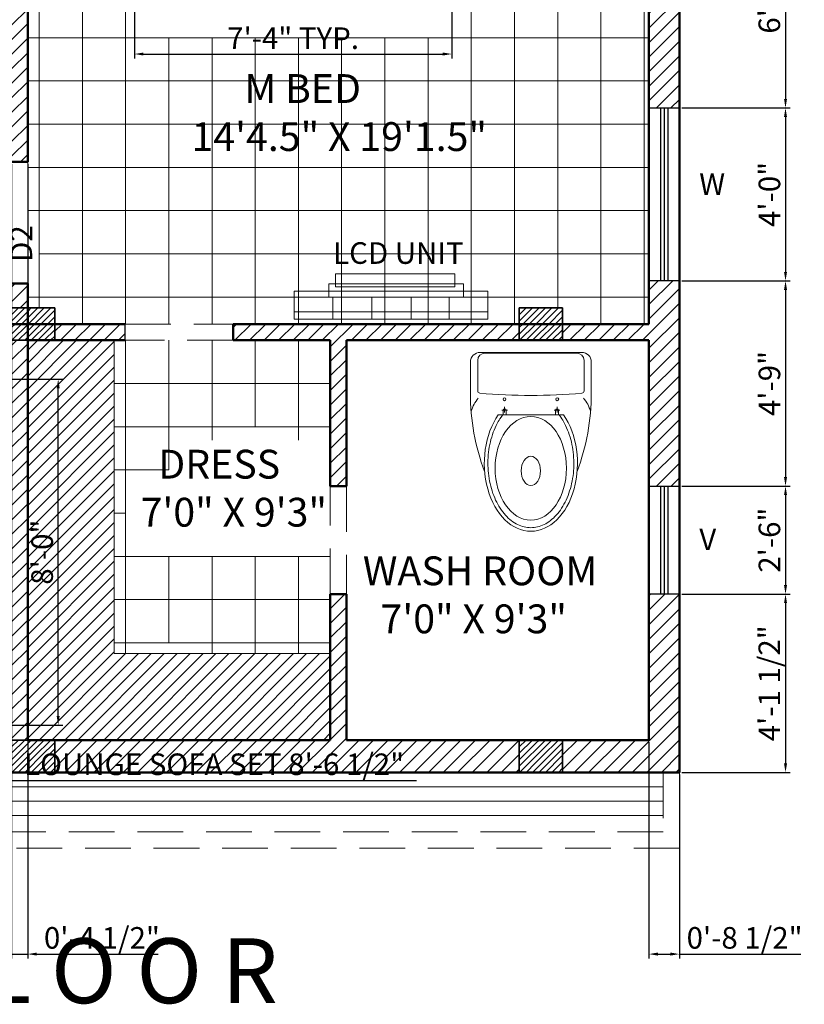
# Model space of a CAD drawing. Units: millimetres. Extents: x 225995 to 227247, y 225507 to 226008.
# Tile 18 of 23: x 227029 to 227247, y 225507 to 225781. Entities that reach past the tile are written whole.
import ezdxf

# ---------------------------------------------------------------- set-up
doc = ezdxf.new("R2010")
doc.units = ezdxf.units.MM
doc.linetypes.add('DASHED', pattern=[19.05, 12.7, -6.35])
for name, color, linetype, lineweight in [('A-ANNO-DIMS', 2, 'Continuous', 18), ('A-ANNO-TEXT', 3, 'Continuous', 18), ('A-AREA-IDEN', 30, 'Continuous', 18), ('A-COLS', 40, 'Continuous', 35), ('A-FLOR-FIXT', 8, 'Continuous', 18), ('A-FLOR-PATT', 8, 'Continuous', 13), ('A-FURN', 9, 'Continuous', 18), ('A-GLAZ', 4, 'Continuous', 25), ('A-WALL', 7, 'Continuous', 50), ('A-WALL-OVHD', 1, 'DASHED', 18), ('A-WALL-PATT', 8, 'Continuous', 13)]:
    doc.layers.add(name, color=color, linetype=linetype, lineweight=lineweight)
doc.styles.get("Standard").update_dxf_attribs({"font": 'arial.ttf'})
doc.dimstyles.new('ISO-25', dxfattribs={"dimtxt": 6, "dimasz": 2.5, "dimexe": 1.25, "dimexo": 0.625, "dimtad": 1, "dimdec": 0, "dimlunit": 3, "dimtxsty": 'Standard', "dimcen": 2.5, "dimadec": 0, "dimazin": 0, "dimtfac": 1, "dimtdec": 0, "dimtmove": 0, "dimatfit": 3, "dimfxl": 1, "dimarcsym": 0})
pattern_1 = [(45, (646.0463, 0.931), (-2.020557627, 2.020557627), [])]
pattern_2 = [(45, (646.0463, 0.931), (-0.898025612, 0.898025612), [])]
pattern_3 = [(45, (787.0463, 0.931), (-0.898025612, 0.898025612), [])]
pattern_4 = [(45, (646.0463, -119.069), (-0.898025612, 0.898025612), [])]
pattern_5 = [(45, (787.0463, -119.069), (-0.898025612, 0.898025612), [])]

# ---------------------------------------------------------------- blocks, each defined once
blk = doc.blocks.new('A$C005B7AE8')
for p, q in [((0.46, 0.74), (0.04, 0.74)), ((0.44, 0.7369), (0.06, 0.7369)), ((0, 0.7), (0, 0.569)), ((0.03, 0.7069), (0.03, 0.5811)), ((0.47, 0.7069), (0.47, 0.5811)), ((0.5, 0.7), (0.5, 0.569)), ((0.1298, 0.5004), (0.1534, 0.5004)), ((0.1356, 0.482), (0.1356, 0.5012)), ((0.1415, 0.4917), (0.1415, 0.5154)), ((0.1478, 0.5012), (0.1478, 0.482)), ((0.3702, 0.5004), (0.3466, 0.5004)), ((0.3522, 0.5012), (0.3522, 0.482)), ((0.3585, 0.4917), (0.3585, 0.5154)), ((0.3644, 0.482), (0.3644, 0.5012)), ((0.3847, 0.482), (0.1153, 0.482))]:
    blk.add_line(p, q)
for centre in [(0.1408, 0.546), (0.3592, 0.546)]:
    blk.add_circle(centre, 0.00582)
for centre, radius, start, end in [((0.04, 0.7), 0.04, 90, 180), ((0.06, 0.7069), 0.03, 90, 180), ((0.44, 0.7069), 0.03, 0, 90), ((0.46, 0.7), 0.04, 0, 90), ((0.9162, 0.5698), 0.9162, 179.9528, 200.6123), ((0.04, 0.5811), 0.01, 180, 265.0115), ((0.25, 2.987), 2.425, 265.0115, 274.9885), ((-0.4162, 0.5698), 0.9162, 339.3877, 0.0472), ((0.46, 0.5811), 0.01, 274.9885, 0), ((0.1538, 0.4498), 0.1579, 140.1815, 162.8478), ((0.3462, 0.4498), 0.1579, 17.1522, 39.8185), ((0.1417, 0.5006), 0.00615, 5.1568, 174.8432), ((0.3583, 0.5006), 0.00615, 5.1568, 174.8432)]:
    blk.add_arc(centre, radius, start, end)
blk.add_ellipse((0.25, 0.281), major_axis=(0, -0.281), ratio=0.685919, start_param=3.915332, end_param=8.651039)
for centre, major_axis, ratio in [((0.2497, 0.2607), (0, -0.2144), 0.687861), ((0.25, 0.2496), (0, -0.0607), 0.657164)]:
    blk.add_ellipse(centre, major_axis=major_axis, ratio=ratio)
blk.add_open_spline([(0.133, 0.4806), (0.1233, 0.4673), (0.1192, 0.4608), (0.109, 0.4431), (0.1032, 0.4313), (0.0931, 0.4064), (0.0887, 0.3933), (0.0814, 0.3662), (0.0785, 0.3521), (0.0743, 0.3236), (0.073, 0.3091), (0.072, 0.2798), (0.0723, 0.2652), (0.0746, 0.2361), (0.0765, 0.2217), (0.0819, 0.1936), (0.0854, 0.1799), (0.0938, 0.1536), (0.0988, 0.141), (0.1099, 0.1171), (0.1162, 0.1059), (0.1297, 0.0851), (0.137, 0.0756), (0.1525, 0.0585), (0.1607, 0.0509), (0.1776, 0.0379), (0.1863, 0.0325), (0.2042, 0.0237), (0.2132, 0.0204), (0.2316, 0.0161), (0.2408, 0.015), (0.2593, 0.015), (0.2685, 0.0161), (0.2868, 0.0205), (0.2959, 0.0237), (0.3137, 0.0325), (0.3225, 0.0379), (0.3394, 0.051), (0.3475, 0.0586), (0.363, 0.0756), (0.3703, 0.0852), (0.3839, 0.1059), (0.3901, 0.1172), (0.4013, 0.141), (0.4062, 0.1537), (0.4146, 0.18), (0.4181, 0.1937), (0.4235, 0.2218), (0.4255, 0.2362), (0.4277, 0.2653), (0.428, 0.2799), (0.427, 0.3091), (0.4257, 0.3237), (0.4215, 0.3522), (0.4186, 0.3662), (0.4113, 0.3933), (0.4069, 0.4064), (0.3967, 0.4313), (0.391, 0.4432), (0.3808, 0.4609), (0.3767, 0.4673), (0.3673, 0.4823)], degree=3, knots=[3.915332, 3.915332, 3.915332, 3.915332, 4.014441, 4.014441, 4.176505, 4.176505, 4.338569, 4.338569, 4.500633, 4.500633, 4.662697, 4.662697, 4.824761, 4.824761, 4.986825, 4.986825, 5.148889, 5.148889, 5.310953, 5.310953, 5.473017, 5.473017, 5.635081, 5.635081, 5.797146, 5.797146, 5.95921, 5.95921, 6.121274, 6.121274, 6.283338, 6.283338, 6.445402, 6.445402, 6.607466, 6.607466, 6.76953, 6.76953, 6.931594, 6.931594, 7.093658, 7.093658, 7.255722, 7.255722, 7.417786, 7.417786, 7.57985, 7.57985, 7.741915, 7.741915, 7.903979, 7.903979, 8.066043, 8.066043, 8.228107, 8.228107, 8.390171, 8.390171, 8.552235, 8.552235, 8.651039, 8.651039, 8.651039, 8.651039])
blk = doc.blocks.new('*D80')
at = {"layer": 'A-ANNO-DIMS', "color": 0, "lineweight": -2, "transparency": 16777216}
for p, q in [((227060.55, 225785.89), (227060.55, 225769.93)), ((227148.66, 225785.89), (227148.66, 225769.93)), ((227063.05, 225771.18), (227146.16, 225771.18))]:
    blk.add_line(p, q, dxfattribs=at)
at = {"layer": 'A-ANNO-DIMS', "color": 0, "transparency": 16777216}
for points in [[(227063.05, 225771.6), (227063.05, 225770.76), (227060.55, 225771.18)], [(227146.16, 225771.6), (227146.16, 225770.76), (227148.66, 225771.18)]]:
    blk.add_solid(points, dxfattribs=at)
at = {"layer": 'Defpoints', "color": 0, "transparency": 16777216}
for p in [(227060.55, 225786.52), (227148.66, 225786.52), (227148.66, 225771.18)]:
    blk.add_point(p, dxfattribs=at)
at = {"layer": 'A-ANNO-DIMS', "color": 0, "transparency": 16777216, "insert": (227104.61, 225774.81), "char_height": 6, "attachment_point": 5}
blk.add_mtext('7\'-4" TYP.', dxfattribs=at)
blk = doc.blocks.new('*D89')
at = {"layer": 'A-ANNO-DIMS', "color": 0, "lineweight": -2, "transparency": 16777216}
for p, q in [((226921.34, 225584.22), (226921.34, 225568.2)), ((227023.97, 225584.22), (227023.97, 225568.2)), ((226923.84, 225569.45), (227021.47, 225569.45)), ((227023.97, 225569.45), (227138.89, 225569.45))]:
    blk.add_line(p, q, dxfattribs=at)
at = {"layer": 'A-ANNO-DIMS', "color": 0, "transparency": 16777216}
for points in [[(226923.84, 225569.87), (226923.84, 225569.03), (226921.34, 225569.45)], [(227021.47, 225569.87), (227021.47, 225569.03), (227023.97, 225569.45)]]:
    blk.add_solid(points, dxfattribs=at)
at = {"layer": 'Defpoints', "color": 0, "transparency": 16777216}
for p in [(226921.34, 225584.85), (227023.97, 225584.85), (227023.97, 225569.45)]:
    blk.add_point(p, dxfattribs=at)
at = {"layer": 'A-ANNO-DIMS', "color": 0, "transparency": 16777216, "insert": (227082.68, 225573.18), "char_height": 6, "attachment_point": 5}
blk.add_mtext('LOUNGE SOFA SET 8\'-6 1/2"', dxfattribs=at)
blk = doc.blocks.new('*D90')
at = {"layer": 'A-ANNO-DIMS', "color": 0, "lineweight": -2, "transparency": 16777216}
for p, q in [((227024.6, 225680.87), (227040.62, 225680.87)), ((227039.37, 225587.35), (227039.37, 225678.37)), ((227024.6, 225584.85), (227040.62, 225584.85))]:
    blk.add_line(p, q, dxfattribs=at)
at = {"layer": 'A-ANNO-DIMS', "color": 0, "transparency": 16777216}
for points in [[(227038.95, 225678.37), (227039.78, 225678.37), (227039.37, 225680.87)], [(227038.95, 225587.35), (227039.78, 225587.35), (227039.37, 225584.85)]]:
    blk.add_solid(points, dxfattribs=at)
at = {"layer": 'Defpoints', "color": 0, "transparency": 16777216}
for p in [(227023.97, 225680.87), (227039.37, 225680.87), (227023.97, 225584.85)]:
    blk.add_point(p, dxfattribs=at)
at = {"layer": 'A-ANNO-DIMS', "color": 0, "transparency": 16777216, "insert": (227035.68, 225632.86), "char_height": 6, "attachment_point": 5, "rotation": 90}
blk.add_mtext('8\'-0"', dxfattribs=at)
blk = doc.blocks.new('*D114')
at = {"layer": 'A-ANNO-DIMS', "color": 0, "lineweight": -2, "transparency": 16777216}
for p, q in [((227203.42, 225580.08), (227203.42, 225520)), ((227211.92, 225571.08), (227211.92, 225520)), ((227205.92, 225521.25), (227209.42, 225521.25)), ((227211.92, 225521.25), (227245.6, 225521.25))]:
    blk.add_line(p, q, dxfattribs=at)
at = {"layer": 'A-ANNO-DIMS', "color": 0, "transparency": 16777216}
for points in [[(227205.92, 225521.67), (227205.92, 225520.84), (227203.42, 225521.25)], [(227209.42, 225521.67), (227209.42, 225520.84), (227211.92, 225521.25)]]:
    blk.add_solid(points, dxfattribs=at)
at = {"layer": 'Defpoints', "color": 0, "transparency": 16777216}
for p in [(227203.42, 225580.7), (227211.92, 225571.7), (227211.92, 225521.25)]:
    blk.add_point(p, dxfattribs=at)
at = {"layer": 'A-ANNO-DIMS', "color": 0, "transparency": 16777216, "insert": (227230.01, 225524.98), "char_height": 6, "attachment_point": 5}
blk.add_mtext('0\'-8 1/2"', dxfattribs=at)
blk = doc.blocks.new('*D115')
at = {"layer": 'A-ANNO-DIMS', "color": 0, "lineweight": -2, "transparency": 16777216}
for p, q in [((227026.42, 225740.58), (227026.42, 225520)), ((227030.92, 225740.58), (227030.92, 225520)), ((227023.92, 225521.25), (227021.42, 225521.25)), ((227026.42, 225521.25), (227030.92, 225521.25)), ((227033.42, 225521.25), (227067.1, 225521.25))]:
    blk.add_line(p, q, dxfattribs=at)
at = {"layer": 'A-ANNO-DIMS', "color": 0, "transparency": 16777216}
for points in [[(227023.92, 225521.67), (227023.92, 225520.84), (227026.42, 225521.25)], [(227033.42, 225521.67), (227033.42, 225520.84), (227030.92, 225521.25)]]:
    blk.add_solid(points, dxfattribs=at)
at = {"layer": 'Defpoints', "color": 0, "transparency": 16777216}
for p in [(227026.42, 225741.2), (227030.92, 225741.2), (227030.92, 225521.25)]:
    blk.add_point(p, dxfattribs=at)
at = {"layer": 'A-ANNO-DIMS', "color": 0, "transparency": 16777216, "insert": (227051.51, 225524.98), "char_height": 6, "attachment_point": 5}
blk.add_mtext('0\'-4 1/2"', dxfattribs=at)
blk = doc.blocks.new('*D126')
at = {"layer": 'A-ANNO-DIMS', "color": 0, "lineweight": -2, "transparency": 16777216}
for p, q in [((227212.55, 225829.7), (227242.62, 225829.7)), ((227241.37, 225827.2), (227241.37, 225758.7)), ((227212.55, 225756.2), (227242.62, 225756.2))]:
    blk.add_line(p, q, dxfattribs=at)
at = {"layer": 'A-ANNO-DIMS', "color": 0, "transparency": 16777216}
for points in [[(227240.96, 225827.2), (227241.79, 225827.2), (227241.37, 225829.7)], [(227240.96, 225758.7), (227241.79, 225758.7), (227241.37, 225756.2)]]:
    blk.add_solid(points, dxfattribs=at)
at = {"layer": 'Defpoints', "color": 0, "transparency": 16777216}
for p in [(227211.92, 225829.7), (227211.92, 225756.2), (227241.37, 225756.2)]:
    blk.add_point(p, dxfattribs=at)
at = {"layer": 'A-ANNO-DIMS', "color": 0, "transparency": 16777216, "insert": (227237.65, 225792.95), "char_height": 6, "attachment_point": 5, "rotation": 90}
blk.add_mtext('6\'-1 1/2"', dxfattribs=at)
blk = doc.blocks.new('*D127')
at = {"layer": 'A-ANNO-DIMS', "color": 0, "lineweight": -2, "transparency": 16777216}
for p, q in [((227212.55, 225756.2), (227242.62, 225756.2)), ((227241.37, 225753.7), (227241.37, 225710.7)), ((227212.55, 225708.2), (227242.62, 225708.2))]:
    blk.add_line(p, q, dxfattribs=at)
at = {"layer": 'A-ANNO-DIMS', "color": 0, "transparency": 16777216}
for points in [[(227240.96, 225753.7), (227241.79, 225753.7), (227241.37, 225756.2)], [(227240.96, 225710.7), (227241.79, 225710.7), (227241.37, 225708.2)]]:
    blk.add_solid(points, dxfattribs=at)
at = {"layer": 'Defpoints', "color": 0, "transparency": 16777216}
for p in [(227211.92, 225756.2), (227211.92, 225708.2), (227241.37, 225708.2)]:
    blk.add_point(p, dxfattribs=at)
at = {"layer": 'A-ANNO-DIMS', "color": 0, "transparency": 16777216, "insert": (227237.68, 225732.2), "char_height": 6, "attachment_point": 5, "rotation": 90}
blk.add_mtext('4\'-0"', dxfattribs=at)
blk = doc.blocks.new('*D128')
at = {"layer": 'A-ANNO-DIMS', "color": 0, "lineweight": -2, "transparency": 16777216}
for p, q in [((227212.55, 225708.2), (227242.62, 225708.2)), ((227241.37, 225705.7), (227241.37, 225653.7)), ((227212.55, 225651.2), (227242.62, 225651.2))]:
    blk.add_line(p, q, dxfattribs=at)
at = {"layer": 'A-ANNO-DIMS', "color": 0, "transparency": 16777216}
for points in [[(227240.96, 225705.7), (227241.79, 225705.7), (227241.37, 225708.2)], [(227240.96, 225653.7), (227241.79, 225653.7), (227241.37, 225651.2)]]:
    blk.add_solid(points, dxfattribs=at)
at = {"layer": 'Defpoints', "color": 0, "transparency": 16777216}
for p in [(227211.92, 225708.2), (227211.92, 225651.2), (227241.37, 225651.2)]:
    blk.add_point(p, dxfattribs=at)
at = {"layer": 'A-ANNO-DIMS', "color": 0, "transparency": 16777216, "insert": (227237.68, 225679.7), "char_height": 6, "attachment_point": 5, "rotation": 90}
blk.add_mtext('4\'-9"', dxfattribs=at)
blk = doc.blocks.new('*D129')
at = {"layer": 'A-ANNO-DIMS', "color": 0, "lineweight": -2, "transparency": 16777216}
for p, q in [((227212.55, 225651.2), (227242.62, 225651.2)), ((227241.37, 225648.7), (227241.37, 225623.7)), ((227212.55, 225621.2), (227242.62, 225621.2))]:
    blk.add_line(p, q, dxfattribs=at)
at = {"layer": 'A-ANNO-DIMS', "color": 0, "transparency": 16777216}
for points in [[(227240.96, 225648.7), (227241.79, 225648.7), (227241.37, 225651.2)], [(227240.96, 225623.7), (227241.79, 225623.7), (227241.37, 225621.2)]]:
    blk.add_solid(points, dxfattribs=at)
at = {"layer": 'Defpoints', "color": 0, "transparency": 16777216}
for p in [(227211.92, 225651.2), (227211.92, 225621.2), (227241.37, 225621.2)]:
    blk.add_point(p, dxfattribs=at)
at = {"layer": 'A-ANNO-DIMS', "color": 0, "transparency": 16777216, "insert": (227237.68, 225636.2), "char_height": 6, "attachment_point": 5, "rotation": 90}
blk.add_mtext('2\'-6"', dxfattribs=at)
blk = doc.blocks.new('*D130')
at = {"layer": 'A-ANNO-DIMS', "color": 0, "lineweight": -2, "transparency": 16777216}
for p, q in [((227212.55, 225621.2), (227242.62, 225621.2)), ((227241.37, 225618.7), (227241.37, 225574.2)), ((227212.55, 225571.7), (227242.62, 225571.7))]:
    blk.add_line(p, q, dxfattribs=at)
at = {"layer": 'A-ANNO-DIMS', "color": 0, "transparency": 16777216}
for points in [[(227240.96, 225618.7), (227241.79, 225618.7), (227241.37, 225621.2)], [(227240.96, 225574.2), (227241.79, 225574.2), (227241.37, 225571.7)]]:
    blk.add_solid(points, dxfattribs=at)
at = {"layer": 'Defpoints', "color": 0, "transparency": 16777216}
for p in [(227211.92, 225621.2), (227211.92, 225571.7), (227241.37, 225571.7)]:
    blk.add_point(p, dxfattribs=at)
at = {"layer": 'A-ANNO-DIMS', "color": 0, "transparency": 16777216, "insert": (227237.65, 225596.45), "char_height": 6, "attachment_point": 5, "rotation": 90}
blk.add_mtext('4\'-1 1/2"', dxfattribs=at)

msp = doc.modelspace()

# ---------------------------------------------------------------- hatches: boundary and pattern name
at = {"layer": 'A-WALL-PATT'}
h = msp.add_hatch(dxfattribs=at)
h.set_pattern_fill('ANSI31', color=256, scale=0.9)
h.set_pattern_definition(pattern_1)
h.paths.add_polyline_path([(227211.92, 225829.7), (227203.42, 225829.7), (227203.42, 225756.2), (227211.92, 225756.2)])
h = msp.add_hatch(dxfattribs=at)
h.set_pattern_fill('ANSI31', color=256, scale=0.9)
h.set_pattern_definition(pattern_1)
h.paths.add_polyline_path([(227030.92, 225809.84), (227026.42, 225809.84), (227026.42, 225741.2), (227030.92, 225741.2)])
h = msp.add_hatch(dxfattribs=at)
h.set_pattern_fill('ANSI31', color=256, scale=0.9)
h.set_pattern_definition(pattern_1)
h.paths.add_polyline_path([(227030.92, 225707.45), (227026.42, 225707.45), (227026.42, 225700.7), (227030.92, 225700.7)])
h = msp.add_hatch(dxfattribs=at)
h.set_pattern_fill('ANSI31', color=256, scale=0.9)
h.set_pattern_definition(pattern_1)
h.paths.add_polyline_path([(227211.92, 225708.2), (227203.42, 225708.2), (227203.42, 225696.2), (227179.42, 225696.2), (227179.42, 225691.7), (227203.42, 225691.7), (227203.42, 225651.2), (227211.92, 225651.2)])
h = msp.add_hatch(dxfattribs=at)
h.set_pattern_fill('ANSI31', color=256, scale=0.4)
h.set_pattern_definition(pattern_2)
h.paths.add_polyline_path([(227030.92, 225700.7), (227026.42, 225700.7), (227026.42, 225696.2), (227030.92, 225696.2)])
h = msp.add_hatch(dxfattribs=at)
h.set_pattern_fill('ANSI31', color=256, scale=0.4)
h.set_pattern_definition(pattern_2)
h.paths.add_polyline_path([(227038.42, 225700.7), (227030.92, 225700.7), (227030.92, 225696.2), (227038.42, 225696.2)])
h = msp.add_hatch(dxfattribs=at)
h.set_pattern_fill('ANSI31', color=256, scale=0.4)
h.set_pattern_definition(pattern_3)
h.paths.add_polyline_path([(227171.92, 225700.7), (227167.42, 225700.7), (227167.42, 225696.2), (227171.92, 225696.2)])
h = msp.add_hatch(dxfattribs=at)
h.set_pattern_fill('ANSI31', color=256, scale=0.4)
h.set_pattern_definition(pattern_3)
h.paths.add_polyline_path([(227179.42, 225700.7), (227171.92, 225700.7), (227171.92, 225696.2), (227179.42, 225696.2)])
h = msp.add_hatch(dxfattribs=at)
h.set_pattern_fill('ANSI31', color=256, scale=0.4)
h.set_pattern_definition(pattern_2)
h.paths.add_polyline_path([(227030.92, 225696.2), (227026.42, 225696.2), (227026.42, 225691.7), (227030.92, 225691.7)])
h = msp.add_hatch(dxfattribs=at)
h.set_pattern_fill('ANSI31', color=256, scale=0.4)
h.set_pattern_definition(pattern_2)
h.paths.add_polyline_path([(227038.42, 225696.2), (227030.92, 225696.2), (227030.92, 225691.7), (227038.42, 225691.7)])
h = msp.add_hatch(dxfattribs=at)
h.set_pattern_fill('ANSI31', color=256, scale=0.9)
h.set_pattern_definition(pattern_1)
h.paths.add_polyline_path([(227057.92, 225696.2), (227038.42, 225696.2), (227038.42, 225691.7), (227057.92, 225691.7)])
h = msp.add_hatch(dxfattribs=at)
h.set_pattern_fill('ANSI31', color=256, scale=0.9)
h.set_pattern_definition(pattern_1)
h.paths.add_polyline_path([(227167.42, 225696.2), (227087.92, 225696.2), (227087.92, 225691.7), (227114.92, 225691.7), (227114.92, 225651.2), (227119.42, 225651.2), (227119.42, 225691.7), (227167.42, 225691.7)])
h = msp.add_hatch(dxfattribs=at)
h.set_pattern_fill('ANSI31', color=256, scale=0.4)
h.set_pattern_definition(pattern_3)
h.paths.add_polyline_path([(227171.92, 225696.2), (227167.42, 225696.2), (227167.42, 225691.7), (227171.92, 225691.7)])
h = msp.add_hatch(dxfattribs=at)
h.set_pattern_fill('ANSI31', color=256, scale=0.4)
h.set_pattern_definition(pattern_3)
h.paths.add_polyline_path([(227179.42, 225696.2), (227171.92, 225696.2), (227171.92, 225691.7), (227179.42, 225691.7)])
h = msp.add_hatch(dxfattribs=at)
h.set_pattern_fill('ANSI31', color=256, scale=0.9)
h.set_pattern_definition(pattern_1)
h.paths.add_polyline_path([(227030.92, 225691.7), (227026.42, 225691.7), (227026.42, 225580.7), (227030.92, 225580.7)])
h = msp.add_hatch(dxfattribs=at)
h.set_pattern_fill('ANSI31', color=256, scale=0.8)
h.set_pattern_definition([(45, (646.0463, 0.931), (-1.796051224, 1.796051224), [])])
h.paths.add_polyline_path([(227114.92, 225604.7), (227054.92, 225604.7), (227054.92, 225691.7), (227030.92, 225691.7), (227030.92, 225580.7), (227038.42, 225580.7), (227114.92, 225580.7)])
h = msp.add_hatch(dxfattribs=at)
h.set_pattern_fill('ANSI31', color=256, scale=0.9)
h.set_pattern_definition(pattern_1)
h.paths.add_polyline_path([(227167.42, 225580.7), (227119.42, 225580.7), (227119.42, 225621.2), (227114.92, 225621.2), (227114.92, 225580.7), (227038.42, 225580.7), (227038.42, 225571.7), (227167.42, 225571.7)])
h = msp.add_hatch(dxfattribs=at)
h.set_pattern_fill('ANSI31', color=256, scale=0.9)
h.set_pattern_definition(pattern_1)
h.paths.add_polyline_path([(227211.92, 225621.2), (227203.42, 225621.2), (227203.42, 225580.7), (227179.42, 225580.7), (227179.42, 225571.7), (227211.92, 225571.7)])
h = msp.add_hatch(dxfattribs=at)
h.set_pattern_fill('ANSI31', color=256, scale=0.4)
h.set_pattern_definition(pattern_4)
h.paths.add_polyline_path([(227030.92, 225580.7), (227026.42, 225580.7), (227026.42, 225576.2), (227030.92, 225576.2)])
h = msp.add_hatch(dxfattribs=at)
h.set_pattern_fill('ANSI31', color=256, scale=0.4)
h.set_pattern_definition(pattern_4)
h.paths.add_polyline_path([(227038.42, 225580.7), (227030.92, 225580.7), (227030.92, 225576.2), (227038.42, 225576.2)])
h = msp.add_hatch(dxfattribs=at)
h.set_pattern_fill('ANSI31', color=256, scale=0.4)
h.set_pattern_definition(pattern_5)
h.paths.add_polyline_path([(227171.92, 225580.7), (227167.42, 225580.7), (227167.42, 225576.2), (227171.92, 225576.2)])
h = msp.add_hatch(dxfattribs=at)
h.set_pattern_fill('ANSI31', color=256, scale=0.4)
h.set_pattern_definition(pattern_5)
h.paths.add_polyline_path([(227179.42, 225580.7), (227171.92, 225580.7), (227171.92, 225576.2), (227179.42, 225576.2)])
h = msp.add_hatch(dxfattribs=at)
h.set_pattern_fill('ANSI31', color=256, scale=0.4)
h.set_pattern_definition(pattern_4)
h.paths.add_polyline_path([(227030.92, 225576.2), (227026.42, 225576.2), (227026.42, 225571.7), (227030.92, 225571.7)])
h = msp.add_hatch(dxfattribs=at)
h.set_pattern_fill('ANSI31', color=256, scale=0.4)
h.set_pattern_definition(pattern_4)
h.paths.add_polyline_path([(227038.42, 225576.2), (227030.92, 225576.2), (227030.92, 225571.7), (227038.42, 225571.7)])
h = msp.add_hatch(dxfattribs=at)
h.set_pattern_fill('ANSI31', color=256, scale=0.4)
h.set_pattern_definition(pattern_5)
h.paths.add_polyline_path([(227171.92, 225576.2), (227167.42, 225576.2), (227167.42, 225571.7), (227171.92, 225571.7)])
h = msp.add_hatch(dxfattribs=at)
h.set_pattern_fill('ANSI31', color=256, scale=0.4)
h.set_pattern_definition(pattern_5)
h.paths.add_polyline_path([(227179.42, 225576.2), (227171.92, 225576.2), (227171.92, 225571.7), (227179.42, 225571.7)])

# ---------------------------------------------------------------- linework, layer by layer
at = {"layer": 'A-ANNO-TEXT'}
msp.add_line((227070.09, 225631.7), (227070.09, 225607.7), dxfattribs=at)
at = {"layer": 'A-COLS'}
for points in [[(227026.42, 225691.7), (227026.42, 225700.7), (227038.42, 225700.7), (227038.42, 225691.7)], [(227167.42, 225691.7), (227167.42, 225700.7), (227179.42, 225700.7), (227179.42, 225691.7)], [(227026.42, 225571.7), (227026.42, 225580.7), (227038.42, 225580.7), (227038.42, 225571.7)], [(227167.42, 225571.7), (227167.42, 225580.7), (227179.42, 225580.7), (227179.42, 225571.7)]]:
    msp.add_lwpolyline(points, close=True, dxfattribs=at)
at = {"layer": 'A-FLOR-PATT'}
for p, q in [((227046.09, 225901.7), (227046.09, 225696.2)), ((227058.09, 225901.7), (227058.09, 225696.2)), ((227154.09, 225901.7), (227154.09, 225696.2)), ((227166.09, 225901.7), (227166.09, 225696.2)), ((227178.09, 225901.7), (227178.09, 225700.7)), ((227190.09, 225901.7), (227190.09, 225696.2)), ((227034.09, 225809.84), (227034.09, 225700.7)), ((227030.92, 225775.7), (227203.42, 225775.7)), ((227070.09, 225775.7), (227070.09, 225696.2)), ((227082.09, 225775.7), (227082.09, 225696.2)), ((227094.09, 225775.7), (227094.09, 225696.2)), ((227106.09, 225775.7), (227106.09, 225696.2)), ((227118.09, 225775.7), (227118.09, 225696.2)), ((227130.09, 225775.7), (227130.09, 225696.2)), ((227142.09, 225775.7), (227142.09, 225696.2)), ((227030.92, 225763.7), (227203.42, 225763.7)), ((227030.92, 225751.7), (227203.42, 225751.7)), ((227030.92, 225739.7), (227203.42, 225739.7)), ((227030.92, 225727.7), (227203.42, 225727.7)), ((227034.09, 225715.7), (227203.42, 225715.7)), ((227030.92, 225703.7), (227203.42, 225703.7)), ((226684.42, 225567.7), (227207.42, 225567.7)), ((226684.42, 225563.7), (227207.42, 225563.7)), ((226684.42, 225559.7), (227207.42, 225559.7))]:
    msp.add_line(p, q, dxfattribs=at)
at = {"layer": 'A-FURN'}
for p, q in [((227202.09, 225901.7), (227202.09, 225696.2)), ((227203.42, 225756.2), (227211.92, 225756.2)), ((227203.42, 225708.2), (227211.92, 225708.2)), ((227115.61, 225703.7), (227115.61, 225697.6)), ((227126.51, 225703.7), (227126.51, 225700.54)), ((227137.37, 225703.7), (227137.37, 225697.6)), ((227147.94, 225703.7), (227147.94, 225697.6)), ((227104.89, 225699.55), (227158.71, 225699.55)), ((227126.51, 225700.54), (227126.51, 225697.6)), ((227038.42, 225696.2), (227057.92, 225696.2)), ((227057.92, 225691.7), (227057.92, 225696.2)), ((227057.92, 225696.2), (227057.92, 225691.7)), ((227057.92, 225691.7), (227038.42, 225691.7)), ((227054.92, 225604.7), (227054.92, 225691.7)), ((227058.09, 225691.7), (227058.09, 225604.7)), ((227070.09, 225691.7), (227070.09, 225655.7)), ((227082.09, 225691.7), (227082.09, 225663.95)), ((227094.09, 225691.7), (227094.09, 225667.7)), ((227106.09, 225691.7), (227106.09, 225663.95)), ((227054.92, 225679.7), (227114.92, 225679.7)), ((227054.92, 225667.7), (227114.92, 225667.7)), ((227054.92, 225655.7), (227070.09, 225655.7)), ((227203.42, 225651.2), (227211.92, 225651.2)), ((227054.92, 225643.7), (227058.09, 225643.7)), ((227054.92, 225631.7), (227114.92, 225631.7)), ((227082.09, 225631.7), (227082.09, 225604.7)), ((227094.09, 225631.7), (227094.09, 225604.7)), ((227106.09, 225631.7), (227106.09, 225604.7)), ((227054.92, 225619.7), (227114.92, 225619.7)), ((227203.42, 225621.2), (227211.92, 225621.2)), ((227054.92, 225607.7), (227114.92, 225607.7)), ((227054.92, 225604.7), (227114.92, 225604.7))]:
    msp.add_line(p, q, dxfattribs=at)
for points in [[(227116.43, 225710.17), (227149.52, 225710.17), (227149.52, 225706.51), (227116.43, 225706.51)], [(227114.55, 225707.4), (227151.97, 225707.4), (227151.97, 225703.7), (227114.55, 225703.7)], [(227104.89, 225705.29), (227158.71, 225705.29), (227158.71, 225697.6), (227104.89, 225697.6)]]:
    msp.add_lwpolyline(points, close=True, dxfattribs=at)
at = {"layer": 'A-GLAZ'}
for p, q in [((227206.67, 225756.2), (227206.67, 225708.2)), ((227207.67, 225756.2), (227207.67, 225708.2)), ((227208.67, 225756.2), (227208.67, 225708.2)), ((227206.67, 225651.2), (227206.67, 225621.2)), ((227207.67, 225651.2), (227207.67, 225621.2)), ((227208.67, 225651.2), (227208.67, 225621.2))]:
    msp.add_line(p, q, dxfattribs=at)
for points in [[(227203.42, 225756.2), (227211.92, 225756.2), (227211.92, 225708.2), (227203.42, 225708.2)], [(227203.42, 225651.2), (227211.92, 225651.2), (227211.92, 225621.2), (227203.42, 225621.2)]]:
    msp.add_lwpolyline(points, close=True, dxfattribs=at)
at = {"layer": 'A-WALL'}
for p, q in [((227211.92, 225934.7), (227211.92, 225571.7)), ((227211.92, 225934.7), (227211.92, 225571.7)), ((227030.92, 225741.2), (227030.92, 225925.7)), ((227030.92, 225925.7), (227030.92, 225741.2)), ((227203.42, 225696.2), (227203.42, 225925.7)), ((227203.42, 225696.2), (227203.42, 225925.7)), ((227026.42, 225741.2), (227030.92, 225741.2)), ((227030.92, 225741.2), (227026.42, 225741.2)), ((227026.42, 225707.45), (227030.92, 225707.45)), ((227026.42, 225707.45), (227030.92, 225707.45)), ((227030.92, 225696.2), (227030.92, 225707.45)), ((227030.92, 225707.45), (227030.92, 225580.7)), ((227026.42, 225696.2), (227057.92, 225696.2)), ((227030.92, 225580.7), (227030.92, 225696.2)), ((227087.92, 225696.2), (227203.42, 225696.2)), ((227087.92, 225691.7), (227087.92, 225696.2)), ((227087.92, 225691.7), (227087.92, 225696.2)), ((227087.92, 225696.2), (227203.42, 225696.2)), ((227030.92, 225691.7), (227057.92, 225691.7)), ((227087.92, 225691.7), (227114.92, 225691.7)), ((227114.92, 225691.7), (227087.92, 225691.7)), ((227114.92, 225651.2), (227114.92, 225691.7)), ((227114.92, 225651.2), (227114.92, 225691.7)), ((227119.42, 225691.7), (227203.42, 225691.7)), ((227119.42, 225651.2), (227119.42, 225691.7)), ((227203.42, 225691.7), (227119.42, 225691.7)), ((227119.42, 225691.7), (227119.42, 225651.2)), ((227203.42, 225580.7), (227203.42, 225691.7)), ((227203.42, 225580.7), (227203.42, 225691.7)), ((227114.92, 225651.2), (227119.42, 225651.2)), ((227119.42, 225651.2), (227114.92, 225651.2)), ((227114.92, 225580.7), (227114.92, 225621.2)), ((227114.92, 225621.2), (227119.42, 225621.2)), ((227114.92, 225580.7), (227114.92, 225621.2)), ((227114.92, 225621.2), (227119.42, 225621.2)), ((227119.42, 225580.7), (227119.42, 225621.2)), ((227119.42, 225621.2), (227119.42, 225580.7)), ((227030.92, 225580.7), (227114.92, 225580.7)), ((227030.92, 225580.7), (227114.92, 225580.7)), ((227119.42, 225580.7), (227203.42, 225580.7)), ((227119.42, 225580.7), (227203.42, 225580.7)), ((227211.92, 225571.7), (226880.92, 225571.7)), ((226990.42, 225571.7), (227211.92, 225571.7))]:
    msp.add_line(p, q, dxfattribs=at)
at = {"layer": 'A-WALL-OVHD'}
for p, q in [((227207.42, 225571.7), (227207.42, 225555.2)), ((227211.92, 225571.7), (227211.92, 225550.7)), ((227207.42, 225555.2), (226684.42, 225555.2)), ((227211.92, 225550.7), (226679.92, 225550.7))]:
    msp.add_line(p, q, dxfattribs=at)
for points in [[(227026.42, 225741.2), (227030.92, 225741.2), (227030.92, 225707.45), (227026.42, 225707.45)], [(227057.97, 225696.2), (227087.92, 225696.2), (227087.92, 225691.7), (227057.97, 225691.7)], [(227114.92, 225651.2), (227119.42, 225651.2), (227119.42, 225621.2), (227114.92, 225621.2)]]:
    msp.add_lwpolyline(points, close=True, dxfattribs=at)

# ---------------------------------------------------------------- block references
at = {"layer": 'A-FLOR-FIXT', "xscale": 67.15513792430541, "yscale": 67.15513792430541, "zscale": 67.15513792430541}
msp.add_blockref('A$C005B7AE8', (227153.86, 225638.65), dxfattribs=at)

# ---------------------------------------------------------------- texts
at = {"layer": 'A-ANNO-TEXT', "attachment_point": 1}
for s, width, insert, char_height in [('   W', 24.8115, (227211.9, 225738.06), 6), ('   LCD UNIT', 85.4795, (227110.22, 225718.92), 6), ('   V', 24.8115, (227211.92, 225639.42), 6), ('D U P L E X  T H I R D  F L O O R', 408.2479, (226763.69, 225525.63), 18)]:
    msp.add_mtext_dynamic_manual_height_columns(s, width=width, gutter_width=12.5, heights=[0], dxfattribs=dict(at, insert=insert, char_height=char_height))
at = {"layer": 'A-ANNO-TEXT', "insert": (227026.14, 225713.45), "char_height": 6, "attachment_point": 1, "rotation": 90}
msp.add_mtext_dynamic_manual_height_columns('D2', width=8.157, gutter_width=12.5, heights=[0], dxfattribs=at)
at = {"layer": 'A-AREA-IDEN', "char_height": 8, "attachment_point": 1}
for s, width, insert in [('        M BED\\P  14\'4.5" X 19\'1.5"', 93.9568, (227071.5, 225765.59)), ('     DRESS\\P   7\'0" X 9\'3"', 85.4795, (227054.92, 225661.29)), (' WASH ROOM\\P   7\'0" X 9\'3"', 85.4795, (227121.55, 225631.68))]:
    msp.add_mtext_dynamic_manual_height_columns(s, width=width, gutter_width=12.5, heights=[0], dxfattribs=dict(at, insert=insert))

# ---------------------------------------------------------------- dimensions: what is measured, and where the dimension line sits
at = {"layer": 'A-ANNO-DIMS'}
for base, p1, p2, override, picture, middle in [((227241.37, 225756.2), (227211.92, 225829.7), (227211.92, 225756.2), {"dimdec": 1, "dimlfac": 1, "dimrnd": 0, "dimzin": 1, "dimdsep": 46, "dimlunit": 4, "dimfrac": 2}, '*D126', (227237.65, 225792.95)), ((227241.37, 225708.2), (227211.92, 225756.2), (227211.92, 225708.2), {"dimdec": 1, "dimlfac": 1, "dimrnd": 0, "dimzin": 1, "dimdsep": 46, "dimlunit": 4, "dimfrac": 2}, '*D127', (227237.68, 225732.2)), ((227241.37, 225651.2), (227211.92, 225708.2), (227211.92, 225651.2), {"dimdec": 1, "dimlfac": 1, "dimrnd": 0, "dimzin": 1, "dimdsep": 46, "dimlunit": 4, "dimfrac": 2}, '*D128', (227237.68, 225679.7)), ((227039.37, 225680.87), (227023.97, 225584.85), (227023.97, 225680.87), {"dimdec": 1, "dimrnd": 0, "dimzin": 1, "dimlunit": 4, "dimfrac": 2}, '*D90', (227035.68, 225632.86)), ((227241.37, 225621.2), (227211.92, 225651.2), (227211.92, 225621.2), {"dimdec": 1, "dimlfac": 1, "dimrnd": 0, "dimzin": 1, "dimdsep": 46, "dimlunit": 4, "dimfrac": 2}, '*D129', (227237.68, 225636.2)), ((227241.37, 225571.7), (227211.92, 225621.2), (227211.92, 225571.7), {"dimdec": 1, "dimlfac": 1, "dimrnd": 0, "dimzin": 1, "dimdsep": 46, "dimlunit": 4, "dimfrac": 2}, '*D130', (227237.65, 225596.45))]:
    dim = msp.add_linear_dim(base=base, p1=p1, p2=p2, angle=90, dimstyle='ISO-25', override=override, dxfattribs=at)
    dim.commit()
    dim.dimension.update_dxf_attribs({"geometry": picture, "text_midpoint": middle})
for base, p1, p2, text, picture, middle in [((227148.66, 225771.18), (227060.55, 225786.52), (227148.66, 225786.52), '<> TYP.', '*D80', (227104.61, 225774.81)), ((227023.97, 225569.45), (226921.34, 225584.85), (227023.97, 225584.85), 'LOUNGE SOFA SET <>', '*D89', (227082.68, 225573.18))]:
    dim = msp.add_linear_dim(base=base, p1=p1, p2=p2, text=text, dimstyle='ISO-25', override={"dimdec": 1, "dimrnd": 0, "dimzin": 1, "dimlunit": 4, "dimfrac": 2}, dxfattribs=at)
    dim.commit()
    dim.dimension.update_dxf_attribs({"geometry": picture, "text_midpoint": middle})
for base, p1, p2, picture, middle in [((227030.92, 225521.25), (227026.42, 225741.2), (227030.92, 225741.2), '*D115', (227051.51, 225524.98)), ((227211.92, 225521.25), (227203.42, 225580.7), (227211.92, 225571.7), '*D114', (227230.01, 225524.98))]:
    dim = msp.add_linear_dim(base=base, p1=p1, p2=p2, dimstyle='ISO-25', override={"dimdec": 1, "dimlfac": 1, "dimrnd": 0, "dimzin": 1, "dimdsep": 46, "dimlunit": 4, "dimfrac": 2}, dxfattribs=at)
    dim.commit()
    dim.dimension.update_dxf_attribs({"geometry": picture, "text_midpoint": middle})

doc.saveas('drawing.dxf')
